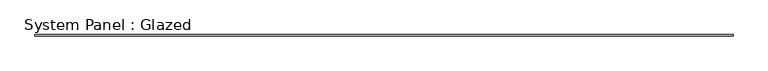
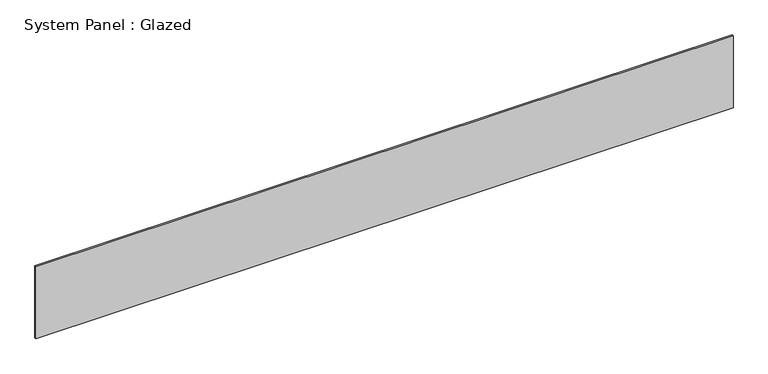
"""IFC4 building model written with IfcOpenShell, lengths in millimetres: plate geometry, System Panel : Glazed."""

from ifc_helpers import new_model, si_unit, origin, origin_with_axes, place, context, project, spatial, polyline, outline, extrude, source, transform, mapped, element, save


def system_panel_glazed_d159b752(model_context):
    return source(origin(), model_context, "Body", "SweptSolid", [
        extrude(outline(polyline([(5584.825, 19.05), (-5584.825, 19.05), (-5584.825, 44.45), (5584.825, 44.45), (5584.825, 19.05)])), origin_with_axes(), (0.0, 0.0, 1.0), 1219.2),
    ])


if __name__ == "__main__":
    model = new_model("IFC4")
    model_context = context("Model", 3, world=origin())
    ifc_project = project(units=[si_unit("LENGTHUNIT", "METRE", prefix="MILLI")], contexts=[model_context])
    site = spatial("IfcSite", under=ifc_project)
    building = spatial("IfcBuilding", under=site)
    placement = place(None, origin())
    system_panel_glazed_shape = system_panel_glazed_d159b752(model_context)
    element("IfcPlate", 1, ObjectType="System Panel : Glazed", at=placement, inside=building, context=model_context, shape_type="MappedRepresentation", body=[
        mapped(system_panel_glazed_shape, transform((0.0, 0.0, 0.0), x_axis=(1.0, 0.0, 0.0), y_axis=(0.0, 1.0, 0.0), z_axis=(0.0, 0.0, 1.0))),
    ])
    save(model, "model.ifc")

# Revit data of these elements
# Type "System Panel : Glazed"
#   Construction Type Id = "GSP4R"
#   Analytic Construction = "1/8 in Pilkington single glazing"
#   Visual Light Transmittance = 0.9
#   Solar Heat Gain Coefficient = 0.86
#   Heat Transfer Coefficient (U) = 1.18115 BTU/(h·ft²·°F)
# Element 1 (IfcPlate, "System Panel : Glazed")
#   Materials on its faces: "Glass"
# Materials
#   "Glass": class "Glass", colour RGB 0 128 192, transparency 0.75, Description = "Soda Lime Glass", Cost = 0
